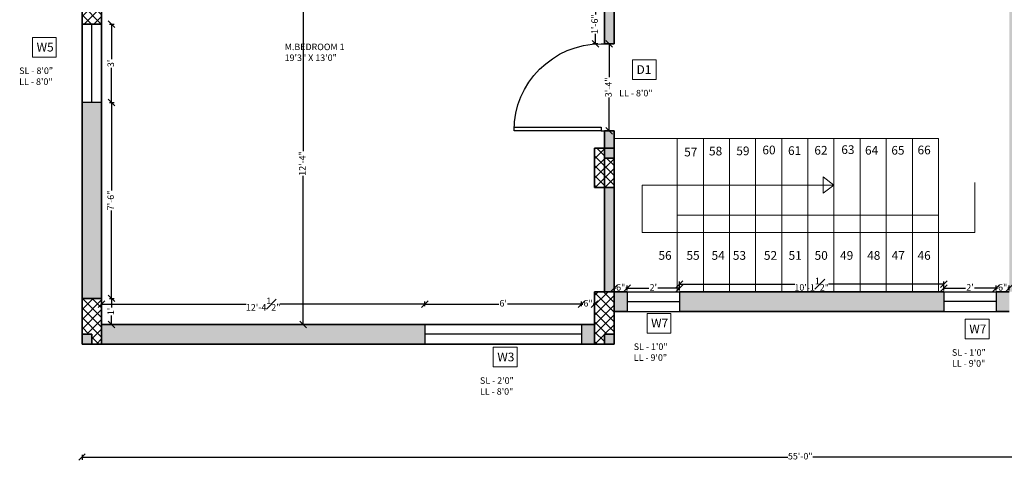
# Model space of a CAD drawing. Units: inches. Extents: x 1365 to 2091, y 1589 to 2091.
# Tile 1 of 8: x 1365 to 1818, y 1589 to 1792. Entities that reach past the tile are written whole.
import ezdxf

# ---------------------------------------------------------------- set-up
doc = ezdxf.new("R2010")
doc.units = ezdxf.units.IN
for name, color, linetype, lineweight in [('A-ANNO-DIMS', 2, 'Continuous', 18), ('A-ANNO-SYMB', 12, 'Continuous', 18), ('A-AREA-IDEN', 7, 'Continuous', 18), ('A-COLS', 7, 'Continuous', 35), ('A-COLS-MARK-PATT', 114, 'Continuous', 13), ('A-COLS-PATT', 1, 'Continuous', 13), ('A-DOOR', 4, 'Continuous', 25), ('A-FLOR-STRS', 254, 'Continuous', 18), ('A-FLOR-STRS-IDEN', 254, 'Continuous', 13), ('A-GLAZ', 150, 'Continuous', 30), ('A-WALL', 7, 'Continuous', 35), ('A-WALL-PATT', 253, 'Continuous', 13)]:
    doc.layers.add(name, color=color, linetype=linetype, lineweight=lineweight)
doc.styles.get("Standard").update_dxf_attribs({"font": 'arial.ttf'})
doc.dimstyles.new('ISO-25', dxfattribs={"dimtxt": 3, "dimasz": 3, "dimexe": 1.25, "dimexo": 0.625, "dimtad": 0, "dimlunit": 4, "dimtxsty": 'Standard', "dimblk": 'OBLIQUE', "dimcen": 2.5, "dimclrd": 254, "dimclre": 254, "dimclrt": 1, "dimadec": 0, "dimazin": 0, "dimtfac": 1, "dimtmove": 0, "dimatfit": 3, "dimfxl": 1, "dimfxlon": 1, "dimfrac": 1, "dimarcsym": 0})

# ---------------------------------------------------------------- blocks, each defined once
blk = doc.blocks.new('*U6')
for p, q in [((0, 0), (0, -6)), ((-40, 0), (-40, -6))]:
    blk.add_line(p, q)
blk.add_lwpolyline([(0, 0), (0, 40), (-1.75, 40), (-1.75, 0)], close=True)
blk.add_arc((0, 0), 40, 90, 180)
blk = doc.blocks.new('_Oblique')
at = {"color": 0, "linetype": 'ByBlock', "lineweight": -2}
blk.add_line((-0.5, -0.5), (0.5, 0.5), dxfattribs=at)
blk = doc.blocks.new('*D41')
at = {"layer": 'A-ANNO-DIMS', "color": 0, "lineweight": -2, "transparency": 16777216}
for p, q in [((1494.36, 1799.86), (1496.61, 1799.86)), ((1495.36, 1799.86), (1495.36, 1731.49)), ((1495.36, 1651.86), (1495.36, 1720.22)), ((1494.36, 1651.86), (1496.61, 1651.86))]:
    blk.add_line(p, q, dxfattribs=at)
at = {"layer": 'Defpoints', "color": 0, "transparency": 16777216}
for p in [(1482.35, 1799.86), (1482.35, 1651.86), (1495.36, 1651.86)]:
    blk.add_point(p, dxfattribs=at)
at = {"layer": 'A-ANNO-DIMS', "color": 0, "lineweight": -2, "transparency": 16777216, "xscale": 3, "yscale": 3, "zscale": 3}
for p, rotation in [((1495.36, 1799.86), 90), ((1495.36, 1651.86), 270)]:
    blk.add_blockref('_Oblique', p, dxfattribs=dict(at, rotation=rotation))
at = {"layer": 'A-ANNO-DIMS', "color": 0, "transparency": 16777216, "insert": (1495.36, 1725.86), "char_height": 3, "attachment_point": 5, "rotation": 90}
blk.add_mtext('12\'-4"', dxfattribs=at)
blk = doc.blocks.new('*D42')
at = {"layer": 'A-ANNO-DIMS', "color": 0, "lineweight": -2, "transparency": 16777216}
for p, q in [((1406.34, 1789.86), (1408.59, 1789.86)), ((1407.34, 1789.86), (1407.34, 1773.86)), ((1407.34, 1753.86), (1407.34, 1769.85)), ((1406.34, 1753.86), (1408.59, 1753.86))]:
    blk.add_line(p, q, dxfattribs=at)
at = {"layer": 'Defpoints', "color": 0, "transparency": 16777216}
for p in [(1402.75, 1789.86), (1402.75, 1753.86), (1407.34, 1753.86)]:
    blk.add_point(p, dxfattribs=at)
at = {"layer": 'A-ANNO-DIMS', "color": 0, "lineweight": -2, "transparency": 16777216, "xscale": 3, "yscale": 3, "zscale": 3}
for p, rotation in [((1407.34, 1789.86), 90), ((1407.34, 1753.86), 270)]:
    blk.add_blockref('_Oblique', p, dxfattribs=dict(at, rotation=rotation))
at = {"layer": 'A-ANNO-DIMS', "color": 0, "transparency": 16777216, "insert": (1407.34, 1771.86), "char_height": 3, "attachment_point": 5, "rotation": 90}
blk.add_mtext("3'", dxfattribs=at)
blk = doc.blocks.new('*D43')
at = {"layer": 'A-ANNO-DIMS', "color": 0, "lineweight": -2, "transparency": 16777216}
for p, q in [((1406.34, 1753.86), (1408.59, 1753.86)), ((1407.34, 1753.86), (1407.34, 1713.46)), ((1407.34, 1663.86), (1407.34, 1704.26)), ((1406.34, 1663.86), (1408.59, 1663.86))]:
    blk.add_line(p, q, dxfattribs=at)
at = {"layer": 'Defpoints', "color": 0, "transparency": 16777216}
for p in [(1402.75, 1753.86), (1402.75, 1663.86), (1407.34, 1663.86)]:
    blk.add_point(p, dxfattribs=at)
at = {"layer": 'A-ANNO-DIMS', "color": 0, "lineweight": -2, "transparency": 16777216, "xscale": 3, "yscale": 3, "zscale": 3}
for p, rotation in [((1407.34, 1753.86), 90), ((1407.34, 1663.86), 270)]:
    blk.add_blockref('_Oblique', p, dxfattribs=dict(at, rotation=rotation))
at = {"layer": 'A-ANNO-DIMS', "color": 0, "transparency": 16777216, "insert": (1407.34, 1708.86), "char_height": 3, "attachment_point": 5, "rotation": 90}
blk.add_mtext('7\'-6"', dxfattribs=at)
blk = doc.blocks.new('*D44')
at = {"layer": 'A-ANNO-DIMS', "color": 0, "lineweight": -2, "transparency": 16777216}
for p, q in [((1406.34, 1663.86), (1408.59, 1663.86)), ((1407.34, 1663.86), (1407.34, 1659.72)), ((1407.34, 1651.86), (1407.34, 1655.99)), ((1406.34, 1651.86), (1408.59, 1651.86))]:
    blk.add_line(p, q, dxfattribs=at)
at = {"layer": 'Defpoints', "color": 0, "transparency": 16777216}
for p in [(1402.75, 1663.86), (1402.75, 1651.86), (1407.34, 1651.86)]:
    blk.add_point(p, dxfattribs=at)
at = {"layer": 'A-ANNO-DIMS', "color": 0, "lineweight": -2, "transparency": 16777216, "xscale": 3, "yscale": 3, "zscale": 3}
for p, rotation in [((1407.34, 1663.86), 90), ((1407.34, 1651.86), 270)]:
    blk.add_blockref('_Oblique', p, dxfattribs=dict(at, rotation=rotation))
at = {"layer": 'A-ANNO-DIMS', "color": 0, "transparency": 16777216, "insert": (1407.34, 1657.86), "char_height": 3, "attachment_point": 5, "rotation": 90}
blk.add_mtext("1'", dxfattribs=at)
blk = doc.blocks.new('*D45')
at = {"layer": 'A-ANNO-DIMS', "color": 0, "lineweight": -2, "transparency": 16777216}
for p, q in [((1402.75, 1660.21), (1402.75, 1662.46)), ((1402.75, 1661.21), (1469.22, 1661.21)), ((1551.25, 1661.21), (1484.79, 1661.21)), ((1551.25, 1660.21), (1551.25, 1662.46))]:
    blk.add_line(p, q, dxfattribs=at)
at = {"layer": 'Defpoints', "color": 0, "transparency": 16777216}
for p in [(1551.25, 1661.21), (1402.75, 1651.86), (1551.25, 1651.86)]:
    blk.add_point(p, dxfattribs=at)
at = {"layer": 'A-ANNO-DIMS', "color": 0, "lineweight": -2, "transparency": 16777216, "xscale": 3, "yscale": 3, "zscale": 3, "rotation": 180}
blk.add_blockref('_Oblique', (1402.75, 1661.21), dxfattribs=at)
at = {"layer": 'A-ANNO-DIMS', "color": 0, "lineweight": -2, "transparency": 16777216, "xscale": 3, "yscale": 3, "zscale": 3}
blk.add_blockref('_Oblique', (1551.25, 1661.21), dxfattribs=at)
at = {"layer": 'A-ANNO-DIMS', "color": 0, "transparency": 16777216, "insert": (1477, 1661.21), "char_height": 3, "attachment_point": 5}
blk.add_mtext('12\'-4{\\H1x;\\S1#2;}"', dxfattribs=at)
blk = doc.blocks.new('*D46')
at = {"layer": 'A-ANNO-DIMS', "color": 0, "lineweight": -2, "transparency": 16777216}
for p, q in [((1551.25, 1660.21), (1551.25, 1662.46)), ((1551.25, 1661.21), (1585.24, 1661.21)), ((1623.25, 1661.21), (1589.27, 1661.21)), ((1623.25, 1660.21), (1623.25, 1662.46))]:
    blk.add_line(p, q, dxfattribs=at)
at = {"layer": 'Defpoints', "color": 0, "transparency": 16777216}
for p in [(1623.25, 1661.21), (1551.25, 1651.86), (1623.25, 1651.86)]:
    blk.add_point(p, dxfattribs=at)
at = {"layer": 'A-ANNO-DIMS', "color": 0, "lineweight": -2, "transparency": 16777216, "xscale": 3, "yscale": 3, "zscale": 3, "rotation": 180}
blk.add_blockref('_Oblique', (1551.25, 1661.21), dxfattribs=at)
at = {"layer": 'A-ANNO-DIMS', "color": 0, "lineweight": -2, "transparency": 16777216, "xscale": 3, "yscale": 3, "zscale": 3}
blk.add_blockref('_Oblique', (1623.25, 1661.21), dxfattribs=at)
at = {"layer": 'A-ANNO-DIMS', "color": 0, "transparency": 16777216, "insert": (1587.25, 1661.21), "char_height": 3, "attachment_point": 5}
blk.add_mtext("6'", dxfattribs=at)
blk = doc.blocks.new('*D47')
at = {"layer": 'A-ANNO-DIMS', "color": 0, "lineweight": -2, "transparency": 16777216}
for p, q in [((1623.25, 1660.21), (1623.25, 1662.46)), ((1623.25, 1661.21), (1623.9, 1661.21)), ((1629.25, 1661.21), (1628.61, 1661.21)), ((1629.25, 1660.21), (1629.25, 1662.46))]:
    blk.add_line(p, q, dxfattribs=at)
at = {"layer": 'Defpoints', "color": 0, "transparency": 16777216}
for p in [(1629.25, 1661.21), (1623.25, 1651.86), (1629.25, 1651.86)]:
    blk.add_point(p, dxfattribs=at)
at = {"layer": 'A-ANNO-DIMS', "color": 0, "lineweight": -2, "transparency": 16777216, "xscale": 3, "yscale": 3, "zscale": 3, "rotation": 180}
blk.add_blockref('_Oblique', (1623.25, 1661.21), dxfattribs=at)
at = {"layer": 'A-ANNO-DIMS', "color": 0, "lineweight": -2, "transparency": 16777216, "xscale": 3, "yscale": 3, "zscale": 3}
blk.add_blockref('_Oblique', (1629.25, 1661.21), dxfattribs=at)
at = {"layer": 'A-ANNO-DIMS', "color": 0, "transparency": 16777216, "insert": (1626.25, 1661.21), "char_height": 3, "attachment_point": 5}
blk.add_mtext('6"', dxfattribs=at)
blk = doc.blocks.new('*D48')
at = {"layer": 'A-ANNO-DIMS', "color": 0, "lineweight": -2, "transparency": 16777216}
for p, q in [((1630.68, 1798.86), (1628.43, 1798.86)), ((1629.68, 1798.86), (1629.68, 1794.33)), ((1629.68, 1780.86), (1629.68, 1785.39)), ((1630.68, 1780.86), (1628.43, 1780.86))]:
    blk.add_line(p, q, dxfattribs=at)
at = {"layer": 'Defpoints', "color": 0, "transparency": 16777216}
for p in [(1633.75, 1798.86), (1629.68, 1780.86), (1633.75, 1780.86)]:
    blk.add_point(p, dxfattribs=at)
at = {"layer": 'A-ANNO-DIMS', "color": 0, "lineweight": -2, "transparency": 16777216, "xscale": 3, "yscale": 3, "zscale": 3}
for p, rotation in [((1629.68, 1798.86), 90), ((1629.68, 1780.86), 270)]:
    blk.add_blockref('_Oblique', p, dxfattribs=dict(at, rotation=rotation))
at = {"layer": 'A-ANNO-DIMS', "color": 0, "transparency": 16777216, "insert": (1629.68, 1789.86), "char_height": 3, "attachment_point": 5, "rotation": 90}
blk.add_mtext('1\'-6"', dxfattribs=at)
blk = doc.blocks.new('*D49')
at = {"layer": 'A-ANNO-DIMS', "color": 0, "lineweight": -2, "transparency": 16777216}
for p, q in [((1636.99, 1780.86), (1634.74, 1780.86)), ((1635.99, 1780.86), (1635.99, 1765.47)), ((1635.99, 1740.86), (1635.99, 1756.25)), ((1636.99, 1740.86), (1634.74, 1740.86))]:
    blk.add_line(p, q, dxfattribs=at)
at = {"layer": 'Defpoints', "color": 0, "transparency": 16777216}
for p in [(1638.25, 1780.86), (1635.99, 1740.86), (1638.25, 1740.86)]:
    blk.add_point(p, dxfattribs=at)
at = {"layer": 'A-ANNO-DIMS', "color": 0, "lineweight": -2, "transparency": 16777216, "xscale": 3, "yscale": 3, "zscale": 3}
for p, rotation in [((1635.99, 1780.86), 90), ((1635.99, 1740.86), 270)]:
    blk.add_blockref('_Oblique', p, dxfattribs=dict(at, rotation=rotation))
at = {"layer": 'A-ANNO-DIMS', "color": 0, "transparency": 16777216, "insert": (1635.99, 1760.86), "char_height": 3, "attachment_point": 5, "rotation": 90}
blk.add_mtext('3\'-4"', dxfattribs=at)
blk = doc.blocks.new('*D50')
at = {"layer": 'A-ANNO-DIMS', "color": 0, "lineweight": -2, "transparency": 16777216}
for p, q in [((1638.25, 1667.5), (1638.25, 1669.75)), ((1644.25, 1667.5), (1644.25, 1669.75)), ((1638.25, 1668.5), (1638.9, 1668.5)), ((1644.25, 1668.5), (1643.61, 1668.5))]:
    blk.add_line(p, q, dxfattribs=at)
at = {"layer": 'Defpoints', "color": 0, "transparency": 16777216}
for p in [(1638.25, 1666.86), (1644.25, 1668.5), (1644.25, 1666.86)]:
    blk.add_point(p, dxfattribs=at)
at = {"layer": 'A-ANNO-DIMS', "color": 0, "lineweight": -2, "transparency": 16777216, "xscale": 3, "yscale": 3, "zscale": 3, "rotation": 180}
blk.add_blockref('_Oblique', (1638.25, 1668.5), dxfattribs=at)
at = {"layer": 'A-ANNO-DIMS', "color": 0, "lineweight": -2, "transparency": 16777216, "xscale": 3, "yscale": 3, "zscale": 3}
blk.add_blockref('_Oblique', (1644.25, 1668.5), dxfattribs=at)
at = {"layer": 'A-ANNO-DIMS', "color": 0, "transparency": 16777216, "insert": (1641.25, 1668.5), "char_height": 3, "attachment_point": 5}
blk.add_mtext('6"', dxfattribs=at)
blk = doc.blocks.new('*D51')
at = {"layer": 'A-ANNO-DIMS', "color": 0, "lineweight": -2, "transparency": 16777216}
for p, q in [((1644.25, 1667.5), (1644.25, 1669.75)), ((1668.25, 1667.5), (1668.25, 1669.75)), ((1644.25, 1668.5), (1654.22, 1668.5)), ((1668.25, 1668.5), (1658.28, 1668.5))]:
    blk.add_line(p, q, dxfattribs=at)
at = {"layer": 'Defpoints', "color": 0, "transparency": 16777216}
for p in [(1644.25, 1666.86), (1668.25, 1668.5), (1668.25, 1666.86)]:
    blk.add_point(p, dxfattribs=at)
at = {"layer": 'A-ANNO-DIMS', "color": 0, "lineweight": -2, "transparency": 16777216, "xscale": 3, "yscale": 3, "zscale": 3, "rotation": 180}
blk.add_blockref('_Oblique', (1644.25, 1668.5), dxfattribs=at)
at = {"layer": 'A-ANNO-DIMS', "color": 0, "lineweight": -2, "transparency": 16777216, "xscale": 3, "yscale": 3, "zscale": 3}
blk.add_blockref('_Oblique', (1668.25, 1668.5), dxfattribs=at)
at = {"layer": 'A-ANNO-DIMS', "color": 0, "transparency": 16777216, "insert": (1656.25, 1668.5), "char_height": 3, "attachment_point": 5}
blk.add_mtext("2'", dxfattribs=at)
blk = doc.blocks.new('*D52')
at = {"layer": 'A-ANNO-DIMS', "color": 0, "lineweight": -2, "transparency": 16777216}
for p, q in [((1789.75, 1667.5), (1789.75, 1669.75)), ((1813.75, 1667.5), (1813.75, 1669.75)), ((1789.75, 1668.5), (1799.72, 1668.5)), ((1813.75, 1668.5), (1803.78, 1668.5))]:
    blk.add_line(p, q, dxfattribs=at)
at = {"layer": 'Defpoints', "color": 0, "transparency": 16777216}
for p in [(1789.75, 1666.86), (1813.75, 1668.5), (1813.75, 1666.86)]:
    blk.add_point(p, dxfattribs=at)
at = {"layer": 'A-ANNO-DIMS', "color": 0, "lineweight": -2, "transparency": 16777216, "xscale": 3, "yscale": 3, "zscale": 3, "rotation": 180}
blk.add_blockref('_Oblique', (1789.75, 1668.5), dxfattribs=at)
at = {"layer": 'A-ANNO-DIMS', "color": 0, "lineweight": -2, "transparency": 16777216, "xscale": 3, "yscale": 3, "zscale": 3}
blk.add_blockref('_Oblique', (1813.75, 1668.5), dxfattribs=at)
at = {"layer": 'A-ANNO-DIMS', "color": 0, "transparency": 16777216, "insert": (1801.75, 1668.5), "char_height": 3, "attachment_point": 5}
blk.add_mtext("2'", dxfattribs=at)
blk = doc.blocks.new('*D53')
at = {"layer": 'A-ANNO-DIMS', "color": 0, "lineweight": -2, "transparency": 16777216}
for p, q in [((1813.75, 1667.5), (1813.75, 1669.75)), ((1819.75, 1667.5), (1819.75, 1669.75)), ((1813.75, 1668.5), (1814.4, 1668.5)), ((1819.75, 1668.5), (1819.11, 1668.5))]:
    blk.add_line(p, q, dxfattribs=at)
at = {"layer": 'Defpoints', "color": 0, "transparency": 16777216}
for p in [(1813.75, 1666.86), (1819.75, 1668.5), (1819.75, 1666.86)]:
    blk.add_point(p, dxfattribs=at)
at = {"layer": 'A-ANNO-DIMS', "color": 0, "lineweight": -2, "transparency": 16777216, "xscale": 3, "yscale": 3, "zscale": 3, "rotation": 180}
blk.add_blockref('_Oblique', (1813.75, 1668.5), dxfattribs=at)
at = {"layer": 'A-ANNO-DIMS', "color": 0, "lineweight": -2, "transparency": 16777216, "xscale": 3, "yscale": 3, "zscale": 3}
blk.add_blockref('_Oblique', (1819.75, 1668.5), dxfattribs=at)
at = {"layer": 'A-ANNO-DIMS', "color": 0, "transparency": 16777216, "insert": (1816.75, 1668.5), "char_height": 3, "attachment_point": 5}
blk.add_mtext('6"', dxfattribs=at)
blk = doc.blocks.new('*D117')
at = {"layer": 'A-ANNO-DIMS', "color": 0, "lineweight": -2, "transparency": 16777216}
for p, q in [((1668.25, 1669.37), (1668.25, 1671.62)), ((1668.25, 1670.37), (1721.22, 1670.37)), ((1789.75, 1670.37), (1736.79, 1670.37)), ((1789.75, 1669.37), (1789.75, 1671.62))]:
    blk.add_line(p, q, dxfattribs=at)
at = {"layer": 'Defpoints', "color": 0, "transparency": 16777216}
for p in [(1789.75, 1670.37), (1668.25, 1666.86), (1789.75, 1666.86)]:
    blk.add_point(p, dxfattribs=at)
at = {"layer": 'A-ANNO-DIMS', "color": 0, "lineweight": -2, "transparency": 16777216, "xscale": 3, "yscale": 3, "zscale": 3, "rotation": 180}
blk.add_blockref('_Oblique', (1668.25, 1670.37), dxfattribs=at)
at = {"layer": 'A-ANNO-DIMS', "color": 0, "lineweight": -2, "transparency": 16777216, "xscale": 3, "yscale": 3, "zscale": 3}
blk.add_blockref('_Oblique', (1789.75, 1670.37), dxfattribs=at)
at = {"layer": 'A-ANNO-DIMS', "color": 0, "transparency": 16777216, "insert": (1729, 1670.37), "char_height": 3, "attachment_point": 5}
blk.add_mtext('10\'-1{\\H1x;\\S1#2;}"', dxfattribs=at)
blk = doc.blocks.new('OPENING-TAG-D1')
blk.add_lwpolyline([(6.13, 13.79), (17.02, 13.79), (17.02, 4.75), (6.13, 4.75)], close=True)
at = {"attachment_point": 1}
for s, width, insert, char_height in [('{D1}', 14.5136, (7.98, 11.34), 4), ('{LL - 8\'0"}', 24.3857, (0, 0), 3)]:
    blk.add_mtext_dynamic_manual_height_columns(s, width=width, gutter_width=12.5, heights=[0], dxfattribs=dict(at, insert=insert, char_height=char_height))
blk = doc.blocks.new('OPENING-TAG-W7')
blk.add_lwpolyline([(6.13, 13.79), (17.02, 13.79), (17.02, 4.75), (6.13, 4.75)], close=True)
at = {"attachment_point": 1}
for s, width, insert, char_height in [('{W7}', 14.5136, (7.98, 11.34), 4), ('{SL - 1\'0"\\PLL - 9\'0"}', 24.3857, (0, 0), 3)]:
    blk.add_mtext_dynamic_manual_height_columns(s, width=width, gutter_width=12.5, heights=[0], dxfattribs=dict(at, insert=insert, char_height=char_height))
blk = doc.blocks.new('*D122')
at = {"layer": 'A-ANNO-DIMS', "color": 254, "lineweight": -2, "transparency": 16777216}
for p, q in [((1393.75, 1591.92), (1393.75, 1589.67)), ((1393.75, 1590.92), (1717.98, 1590.92)), ((2053.75, 1590.92), (1729.53, 1590.92)), ((2053.75, 1591.92), (2053.75, 1589.67))]:
    blk.add_line(p, q, dxfattribs=at)
at = {"layer": 'Defpoints', "color": 0, "transparency": 16777216}
for p in [(1393.75, 1642.86), (2053.75, 1642.86), (2053.75, 1590.92)]:
    blk.add_point(p, dxfattribs=at)
at = {"layer": 'A-ANNO-DIMS', "color": 254, "lineweight": -2, "transparency": 16777216, "xscale": 3, "yscale": 3, "zscale": 3, "rotation": 180}
blk.add_blockref('_Oblique', (1393.75, 1590.92), dxfattribs=at)
at = {"layer": 'A-ANNO-DIMS', "color": 254, "lineweight": -2, "transparency": 16777216, "xscale": 3, "yscale": 3, "zscale": 3}
blk.add_blockref('_Oblique', (2053.75, 1590.92), dxfattribs=at)
at = {"layer": 'A-ANNO-DIMS', "color": 1, "transparency": 16777216, "insert": (1723.75, 1590.92), "char_height": 3, "attachment_point": 5}
blk.add_mtext('55\'-0"', dxfattribs=at)

msp = doc.modelspace()

# ---------------------------------------------------------------- hatches: boundary and pattern name
at = {"layer": 'A-COLS-MARK-PATT'}
h = msp.add_hatch(color=256, dxfattribs=at)
h.dxf.hatch_style = 1
h.paths.add_polyline_path([(1398.254, 2062.858), (1393.754, 2062.858), (1393.754, 2058.358), (1398.254, 2058.358)])
h.paths.add_polyline_path([(1398.254, 1872.358), (1393.754, 1872.358), (1393.754, 1867.858), (1398.254, 1867.858)])
h.paths.add_polyline_path([(1398.254, 1807.858), (1393.754, 1807.858), (1393.754, 1803.358), (1398.254, 1803.358)])
h.paths.add_polyline_path([(1398.254, 1647.358), (1393.754, 1647.358), (1393.754, 1642.858), (1398.254, 1642.858)])
h.paths.add_polyline_path([(1638.254, 1647.358), (1633.754, 1647.358), (1633.754, 1642.858), (1638.254, 1642.858)])
h.paths.add_polyline_path([(1638.254, 1732.858), (1633.754, 1732.858), (1633.754, 1728.358), (1638.254, 1728.358)])
h.paths.add_polyline_path([(1647.254, 1876.858), (1642.754, 1876.858), (1642.754, 1872.358), (1647.254, 1872.358)])
h.paths.add_polyline_path([(1647.254, 1803.358), (1642.754, 1803.358), (1642.754, 1798.858), (1647.254, 1798.858)])
h.paths.add_polyline_path([(1647.254, 2062.858), (1642.754, 2062.858), (1642.754, 2058.358), (1647.254, 2058.358)])
h.paths.add_polyline_path([(1824.254, 2062.858), (1819.754, 2062.858), (1819.754, 2058.358), (1824.254, 2058.358)])
h.paths.add_polyline_path([(1824.254, 1885.858), (1819.754, 1885.858), (1819.754, 1881.358), (1824.254, 1881.358)])
h.paths.add_polyline_path([(1828.754, 1647.358), (1824.254, 1647.358), (1824.254, 1642.858), (1828.754, 1642.858)])
h.paths.add_polyline_path([(1948.754, 1647.358), (1944.254, 1647.358), (1944.254, 1642.858), (1948.754, 1642.858)])
h.paths.add_polyline_path([(2041.754, 1647.358), (2037.254, 1647.358), (2037.254, 1642.858), (2041.754, 1642.858)])
h.paths.add_polyline_path([(2041.754, 1885.858), (2037.254, 1885.858), (2037.254, 1881.358), (2041.754, 1881.358)])
h.paths.add_polyline_path([(2041.754, 2062.858), (2037.254, 2062.858), (2037.254, 2058.358), (2041.754, 2058.358)])
at = {"layer": 'A-COLS-PATT'}
h = msp.add_hatch(dxfattribs=at)
h.set_pattern_fill('ANSI37', color=256)
h.paths.add_polyline_path([(1414.754, 2062.858), (1398.254, 2062.858), (1398.254, 2058.358), (1393.754, 2058.358), (1393.754, 2053.858), (1414.754, 2053.858)])
h.paths.add_polyline_path([(1402.754, 1888.858), (1393.754, 1888.858), (1393.754, 1872.358), (1398.254, 1872.358), (1398.254, 1867.858), (1402.754, 1867.858), (1402.754, 1872.358)])
h.paths.add_polyline_path([(1402.754, 1807.858), (1398.254, 1807.858), (1398.254, 1803.358), (1393.754, 1803.358), (1393.754, 1789.858), (1402.754, 1789.858)])
h.paths.add_polyline_path([(1402.754, 1663.858), (1393.754, 1663.858), (1393.754, 1647.358), (1398.254, 1647.358), (1398.254, 1642.858), (1402.754, 1642.858)])
h.paths.add_polyline_path([(1638.254, 1666.858), (1629.254, 1666.858), (1629.254, 1642.858), (1633.754, 1642.858), (1633.754, 1647.358), (1638.254, 1647.358)])
h.paths.add_polyline_path([(1633.754, 1732.858), (1629.254, 1732.858), (1629.254, 1714.858), (1633.754, 1714.858)])
h.paths.add_polyline_path([(1638.254, 1728.358), (1633.754, 1728.358), (1633.754, 1714.858), (1638.254, 1714.858)])
at = {"layer": 'A-WALL-PATT'}
h = msp.add_hatch(color=256, dxfattribs=at)
h.dxf.hatch_style = 1
h.paths.add_polyline_path([(1638.254, 2053.858), (1638.254, 2062.858), (1617.254, 2062.858), (1617.254, 2053.858)])
h.paths.add_polyline_path([(1633.754, 1780.858), (1638.254, 1780.858), (1638.254, 1798.858), (1633.754, 1798.858)])
h.paths.add_polyline_path([(1828.754, 2038.858), (1819.754, 2038.858), (1819.754, 1925.829), (1828.754, 1925.829)])
h = msp.add_hatch(color=256, dxfattribs=at)
h.dxf.hatch_style = 1
h.paths.add_polyline_path([(1402.754, 1753.858), (1393.754, 1753.858), (1393.754, 1663.858), (1402.754, 1663.858)])
h.paths.add_polyline_path([(1533.254, 1804.358), (1476.254, 1804.358), (1476.254, 1816.358), (1471.754, 1816.358), (1471.754, 1804.358), (1402.754, 1804.358), (1402.754, 1799.858), (1533.254, 1799.858)])
h.paths.add_polyline_path([(1638.254, 1714.858), (1633.754, 1714.858), (1633.754, 1666.858), (1638.254, 1666.858)])
h.paths.add_polyline_path([(1638.254, 1740.858), (1633.754, 1740.858), (1633.754, 1732.858), (1638.254, 1732.858)])
h.paths.add_polyline_path([(1954.754, 1744.858), (1948.754, 1744.858), (1944.254, 1744.858), (1824.254, 1744.858), (1824.254, 1821.858), (1819.754, 1821.858), (1819.754, 1666.858), (1824.254, 1666.858), (1824.254, 1740.358), (1944.254, 1740.358), (1948.754, 1740.358), (1954.754, 1740.358)])
h.paths.add_polyline_path([(1948.754, 1698.358), (1944.254, 1698.358), (1944.254, 1651.858), (1948.754, 1651.858)])
h.paths.add_polyline_path([(1948.754, 1740.358), (1944.254, 1740.358), (1944.254, 1734.358), (1948.754, 1734.358)], flags=17)
h = msp.add_hatch(color=256, dxfattribs=at)
h.dxf.hatch_style = 1
h.paths.add_polyline_path([(1789.754, 1666.858), (1668.254, 1666.858), (1668.254, 1657.858), (1789.754, 1657.858)])
h.paths.add_polyline_path([(1644.254, 1666.858), (1638.254, 1666.858), (1638.254, 1657.858), (1644.254, 1657.858)])
h.paths.add_polyline_path([(1819.754, 1666.858), (1813.754, 1666.858), (1813.754, 1657.858), (1819.754, 1657.858)])
h = msp.add_hatch(color=256, dxfattribs=at)
h.dxf.hatch_style = 1
h.paths.add_polyline_path([(1551.254, 1651.858), (1402.754, 1651.858), (1402.754, 1642.858), (1551.254, 1642.858)])
h.paths.add_polyline_path([(1629.254, 1651.858), (1623.254, 1651.858), (1623.254, 1642.858), (1629.254, 1642.858)])

# ---------------------------------------------------------------- linework, layer by layer
at = {"layer": 'A-ANNO-SYMB'}
for points in [[(1371.061, 1783.76), (1381.95, 1783.76), (1381.95, 1774.722), (1371.061, 1774.722)], [(1582.734, 1641.353), (1593.623, 1641.353), (1593.623, 1632.316), (1582.734, 1632.316)]]:
    msp.add_lwpolyline(points, close=True, dxfattribs=at)
at = {"layer": 'A-COLS'}
for p, q in [((1402.754, 1789.858), (1393.754, 1789.858)), ((1633.754, 1732.858), (1629.254, 1732.858)), ((1629.254, 1732.858), (1629.254, 1714.858)), ((1638.254, 1732.858), (1633.754, 1732.858)), ((1638.254, 1732.858), (1638.254, 1728.358)), ((1638.254, 1728.358), (1633.754, 1728.358)), ((1629.254, 1714.858), (1638.254, 1714.858)), ((1638.254, 1666.858), (1629.254, 1666.858)), ((1629.254, 1666.858), (1629.254, 1642.858)), ((1402.754, 1663.858), (1393.754, 1663.858)), ((1393.754, 1642.858), (1393.754, 1647.358)), ((1393.754, 1647.358), (1398.254, 1647.358)), ((1398.254, 1647.358), (1398.254, 1642.858)), ((1633.754, 1647.358), (1633.754, 1642.858)), ((1633.754, 1647.358), (1638.254, 1647.358))]:
    msp.add_line(p, q, dxfattribs=at)
at = {"layer": 'A-FLOR-STRS'}
for p, q in [((1638.254, 1737.276), (1787.254, 1737.276)), ((1667.254, 1737.276), (1667.254, 1666.858)), ((1679.254, 1737.276), (1679.254, 1666.858)), ((1691.254, 1737.276), (1691.254, 1666.858)), ((1703.254, 1737.276), (1703.254, 1666.858)), ((1715.254, 1737.276), (1715.254, 1666.858)), ((1727.254, 1737.276), (1727.254, 1666.858)), ((1739.254, 1737.276), (1739.254, 1666.858)), ((1751.254, 1737.276), (1751.254, 1666.858)), ((1763.254, 1737.276), (1763.254, 1666.858)), ((1775.254, 1737.276), (1775.254, 1666.858)), ((1787.254, 1737.276), (1787.254, 1666.858)), ((1787.254, 1702.067), (1667.254, 1702.067))]:
    msp.add_line(p, q, dxfattribs=at)
at = {"layer": 'A-FLOR-STRS-IDEN'}
for p, q in [((1739.254, 1715.897), (1734.351, 1719.754)), ((1734.351, 1719.754), (1734.351, 1712.137)), ((1651.081, 1694.083), (1651.081, 1715.897)), ((1651.081, 1715.897), (1739.254, 1715.897)), ((1734.351, 1712.137), (1739.254, 1715.897)), ((1803.966, 1717.045), (1803.966, 1694.083)), ((1803.966, 1694.083), (1651.081, 1694.083))]:
    msp.add_line(p, q, dxfattribs=at)
at = {"layer": 'A-GLAZ'}
for p, q in [((1398.254, 1753.858), (1398.254, 1789.858)), ((1402.754, 1753.858), (1393.754, 1753.858)), ((1644.254, 1666.858), (1668.254, 1666.858)), ((1644.254, 1666.858), (1644.254, 1657.858)), ((1668.254, 1666.858), (1668.254, 1657.858)), ((1789.754, 1666.858), (1813.754, 1666.858)), ((1789.754, 1666.858), (1789.754, 1657.858)), ((1813.754, 1666.858), (1813.754, 1657.858)), ((1644.254, 1662.358), (1668.254, 1662.358)), ((1813.754, 1662.358), (1789.754, 1662.358)), ((1644.254, 1657.858), (1668.254, 1657.858)), ((1789.754, 1657.858), (1813.754, 1657.858)), ((1551.254, 1651.858), (1551.254, 1642.858)), ((1623.254, 1651.858), (1623.254, 1642.858)), ((1623.254, 1647.358), (1551.254, 1647.358))]:
    msp.add_line(p, q, dxfattribs=at)
at = {"layer": 'A-WALL'}
for p, q in [((1393.754, 1642.858), (1393.754, 2062.858)), ((1402.754, 1642.858), (1402.754, 1807.858)), ((1633.754, 1780.858), (1633.754, 1798.858)), ((1638.254, 1798.858), (1638.254, 1780.858)), ((1638.254, 1780.858), (1633.754, 1780.858)), ((1638.254, 1740.858), (1633.754, 1740.858)), ((1633.754, 1740.858), (1633.754, 1666.858)), ((1638.254, 1740.858), (1638.254, 1642.858)), ((1638.254, 1666.858), (1644.254, 1666.858)), ((1668.254, 1666.858), (1789.754, 1666.858)), ((1813.754, 1666.858), (1819.754, 1666.858)), ((1638.254, 1657.858), (1644.254, 1657.858)), ((1668.254, 1657.858), (1789.754, 1657.858)), ((1813.754, 1657.858), (1819.754, 1657.858)), ((1402.754, 1651.858), (1629.254, 1651.858)), ((1393.754, 1642.858), (1638.254, 1642.858))]:
    msp.add_line(p, q, dxfattribs=at)

# ---------------------------------------------------------------- block references
at = {"layer": 'A-ANNO-SYMB'}
for name, p in [('OPENING-TAG-D1', (1640.579, 1759.685)), ('OPENING-TAG-W7', (1647.258, 1643.134)), ('OPENING-TAG-W7', (1793.453, 1640.468))]:
    msp.add_blockref(name, p, dxfattribs=at)
at = {"layer": 'A-DOOR', "xscale": -1, "rotation": 90}
msp.add_blockref('*U6', (1632.254, 1740.858), dxfattribs=at)

# ---------------------------------------------------------------- texts
at = {"layer": 'A-ANNO-SYMB', "attachment_point": 1}
for s, width, insert, char_height in [('{W5}', 14.51356, (1372.901, 1781.309), 4), ('{SL - 8\'0"\\PLL - 8\'0"}', 24.3857, (1364.926, 1769.974), 3), ('{W3}', 14.51356, (1584.575, 1638.902), 4), ('{SL - 2\'0"\\PLL - 8\'0"}', 24.3857, (1576.599, 1627.567), 3)]:
    msp.add_mtext_dynamic_manual_height_columns(s, width=width, gutter_width=12.5, heights=[0], dxfattribs=dict(at, insert=insert, char_height=char_height))
at = {"layer": 'A-AREA-IDEN', "insert": (1486.862, 1780.946), "char_height": 3, "attachment_point": 1}
msp.add_mtext_dynamic_manual_height_columns('{M.BEDROOM 1\\P19\'3" X 13\'0"}', width=33.58604, gutter_width=12.5, heights=[0], dxfattribs=at)
at = {"layer": 'A-FLOR-STRS-IDEN', "char_height": 4, "attachment_point": 1}
for s, insert in [('57', (1670.431, 1733.11)), ('58', (1681.821, 1733.559)), ('59', (1694.38, 1733.647)), ('60', (1706.353, 1734.061)), ('61', (1718.143, 1733.763)), ('62', (1730.232, 1733.912)), ('63', (1742.619, 1734.21)), ('64', (1753.514, 1733.912)), ('65', (1765.602, 1733.912)), ('66', (1777.631, 1734.055)), ('56', (1658.599, 1685.582)), ('55', (1671.458, 1685.582)), ('54', (1683.007, 1685.582)), ('53', (1692.787, 1685.582)), ('52', (1707.072, 1685.582)), ('51', (1718.387, 1685.582)), ('50', (1730.352, 1685.582)), ('49', (1742.039, 1685.582)), ('48', (1754.497, 1685.582)), ('47', (1765.741, 1685.582)), ('46', (1777.631, 1685.582))]:
    msp.add_mtext_dynamic_manual_height_columns(s, width=7.6501, gutter_width=12.5, heights=[0], dxfattribs=dict(at, insert=insert))

# ---------------------------------------------------------------- dimensions: what is measured, and where the dimension line sits
at = {"layer": 'A-ANNO-DIMS'}
for base, p1, p2, override, picture, middle in [((1495.361, 1651.858), (1482.353, 1799.858), (1482.353, 1651.858), {"dimclrd": 0, "dimclre": 0, "dimclrt": 0}, '*D41', (1495.361, 1725.858)), ((1629.681, 1780.858), (1633.754, 1798.858), (1633.754, 1780.858), {"dimclrd": 0, "dimclre": 0, "dimclrt": 0}, '*D48', (1629.681, 1789.858)), ((1407.337, 1753.858), (1402.754, 1789.858), (1402.754, 1753.858), {"dimclrd": 0, "dimclre": 0, "dimclrt": 0}, '*D42', (1407.337, 1771.858)), ((1635.99, 1740.858), (1638.254, 1780.858), (1638.254, 1740.858), {"dimclrd": 0, "dimclre": 0, "dimclrt": 0}, '*D49', (1635.99, 1760.858)), ((1407.337, 1663.858), (1402.754, 1753.858), (1402.754, 1663.858), {"dimclrd": 0, "dimclre": 0, "dimclrt": 0, "dimtmove": 1}, '*D43', (1407.337, 1708.858)), ((1407.337, 1651.858), (1402.754, 1663.858), (1402.754, 1651.858), {"dimclrd": 0, "dimclre": 0, "dimclrt": 0, "dimtmove": 1}, '*D44', (1407.337, 1657.858))]:
    dim = msp.add_linear_dim(base=base, p1=p1, p2=p2, angle=90, dimstyle='ISO-25', override=override, dxfattribs=at)
    dim.commit()
    dim.dimension.update_dxf_attribs({"geometry": picture, "text_midpoint": middle})
for base, p1, p2, override, picture, middle in [((1644.254, 1668.5), (1638.254, 1666.858), (1644.254, 1666.858), {"dimclrd": 0, "dimclre": 0, "dimclrt": 0}, '*D50', (1641.254, 1668.5)), ((1668.254, 1668.5), (1644.254, 1666.858), (1668.254, 1666.858), {"dimclrd": 0, "dimclre": 0, "dimclrt": 0, "dimtmove": 1}, '*D51', (1656.254, 1668.5)), ((1813.754, 1668.5), (1789.754, 1666.858), (1813.754, 1666.858), {"dimclrd": 0, "dimclre": 0, "dimclrt": 0, "dimtmove": 1}, '*D52', (1801.754, 1668.5)), ((1819.754, 1668.5), (1813.754, 1666.858), (1819.754, 1666.858), {"dimclrd": 0, "dimclre": 0, "dimclrt": 0, "dimtmove": 1}, '*D53', (1816.754, 1668.5)), ((1551.254, 1661.206), (1402.754, 1651.858), (1551.254, 1651.858), {"dimclrd": 0, "dimclre": 0, "dimclrt": 0}, '*D45', (1477.004, 1661.206)), ((1623.254, 1661.206), (1551.254, 1651.858), (1623.254, 1651.858), {"dimclrd": 0, "dimclre": 0, "dimclrt": 0, "dimtmove": 1}, '*D46', (1587.254, 1661.206)), ((1629.254, 1661.206), (1623.254, 1651.858), (1629.254, 1651.858), {"dimclrd": 0, "dimclre": 0, "dimclrt": 0, "dimtmove": 1}, '*D47', (1626.254, 1661.206)), ((2053.754, 1590.921), (1393.754, 1642.858), (2053.754, 1642.858), {"dimdec": 1, "dimlfac": 1, "dimrnd": 0, "dimzin": 1, "dimdsep": 46, "dimlunit": 4, "dimfrac": 2}, '*D122', (1723.754, 1590.921))]:
    dim = msp.add_linear_dim(base=base, p1=p1, p2=p2, dimstyle='ISO-25', override=override, dxfattribs=at)
    dim.commit()
    dim.dimension.update_dxf_attribs({"geometry": picture, "text_midpoint": middle})
dim = msp.add_linear_dim(base=(1789.754, 1670.368), p1=(1668.254, 1666.858), p2=(1789.754, 1666.858), dimstyle='ISO-25', override={"dimclrd": 0, "dimclre": 0, "dimclrt": 0}, dxfattribs=at)
dim.commit()
dim.dimension.update_dxf_attribs({"geometry": '*D117', "text_midpoint": (1729.004, 1670.368), "dimtype": 160})

doc.saveas('drawing.dxf')
